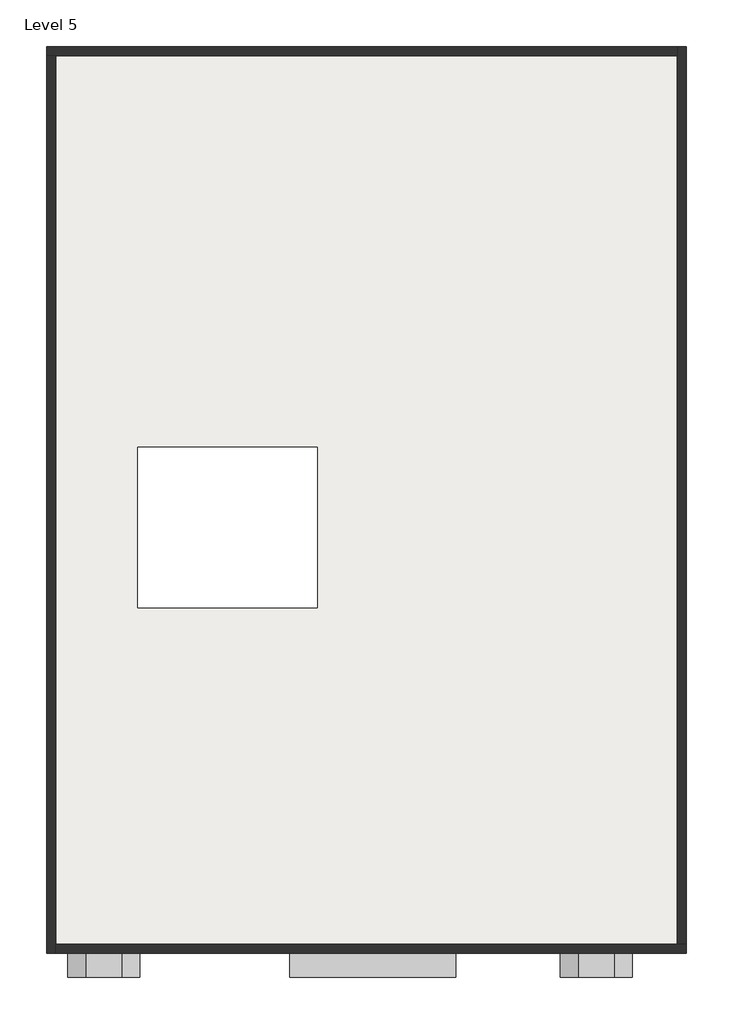
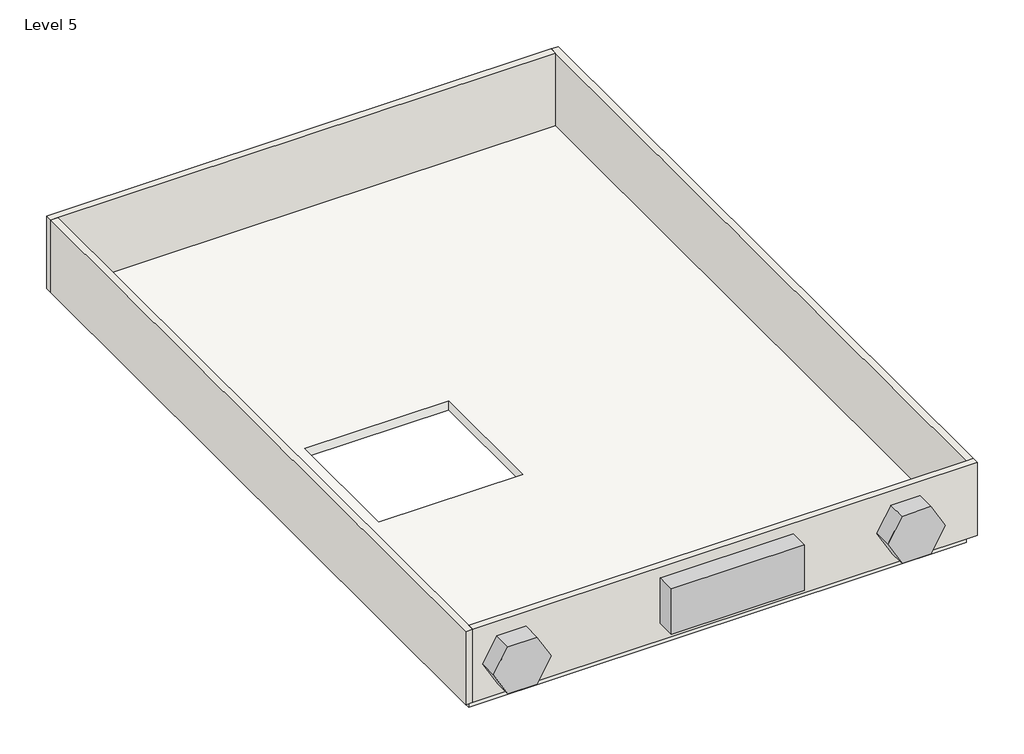
# One storey: 4 walls, 1 proxy, 1 roof.
"""IFC4 building model written with IfcOpenShell, lengths in millimetres."""

from ifc_helpers import new_model, si_unit, frame, origin, place, context, project, spatial, polyline, outline, extrude, faceted_brep, transform, mapped, element, save
from components import generic_models_1_generic_models_1_074ece3c

model = new_model("IFC4")

# Units and contexts
model_context = context("Model", 3, world=origin())
ifc_project = project(units=[si_unit("LENGTHUNIT", "METRE", prefix="MILLI")], contexts=[model_context])

# Site, building, storey
site = spatial("IfcSite", under=ifc_project)
building = spatial("IfcBuilding", under=site)
storey = spatial("IfcBuildingStorey", under=building, Name="Level 5", Elevation=9601.2)

# Proxy
placement = place(None, origin())
generic_models_1_generic_models_1_shape = generic_models_1_generic_models_1_074ece3c(model_context)
element("IfcBuildingElementProxy", 1, Name="Generic Models 1 : Generic Models 1", ObjectType="Generic Models 1 : Generic Models 1", at=placement, inside=storey, context=model_context, shape_type="MappedRepresentation", body=[
    mapped(generic_models_1_generic_models_1_shape, transform((0.0, 0.0, 0.0), x_axis=(1.0, 0.0, 0.0), y_axis=(0.0, 1.0, 0.0), z_axis=(0.0, 0.0, 1.0))),
])

# Roof
element("IfcRoof", 2, ObjectType="Generic - 12\"", at=placement, inside=storey, context=model_context, shape_type="SweptSolid", body=[
    extrude(outline(polyline([(-5216.1449167, -5508.2570853), (-5216.1449167, 5769.3429147), (2670.5550833, 5769.3429147), (2670.5550833, -5508.2570853), (-5216.1449167, -5508.2570853)]), holes=[polyline([(-1894.5382248, 797.2929147), (-4174.7449167, 797.2929147), (-4174.7449167, -1234.7070853), (-1894.5382248, -1234.7070853), (-1894.5382248, 797.2929147)])]), frame((0.0, 0.0, 9448.8), z_axis=(0.0, 0.0, 1.0), x_axis=(1.0, 0.0, 0.0)), (0.0, 0.0, 1.0), 152.4),
])

# Walls
element("IfcWall", 3, ObjectType="WALL4.5\"", at=placement, inside=storey, context=model_context, shape_type="Brep", body=[
    faceted_brep([(-5330.4449167, 5769.3429147, 9601.2), (-5216.1449167, 5769.3429147, 9601.2), (2670.5550833, 5769.3429147, 9601.2), (2670.5550833, 5769.3429147, 10820.4), (-5216.1449167, 5769.3429147, 10820.4), (-5330.4449167, 5769.3429147, 10820.4), (-5330.4449167, 5883.6429147, 9601.2), (-5330.4449167, 5883.6429147, 10820.4), (2670.5550833, 5883.6429147, 10820.4), (2670.5550833, 5883.6429147, 9601.2)], [[[0, 1, 2, 3, 4, 5]], [[6, 7, 8, 9]], [[2, 1, 0, 6, 9]], [[5, 4, 3, 8, 7]], [[0, 5, 7, 6]], [[3, 2, 9, 8]]]),
])
element("IfcWall", 4, ObjectType="WALL4.5\"", at=placement, inside=storey, context=model_context, shape_type="Brep", body=[
    faceted_brep([(-5216.1449167, -5622.5570853, 9601.2), (-5216.1449167, -5508.2570853, 9601.2), (-5216.1449167, 5769.3429147, 9601.2), (-5216.1449167, 5769.3429147, 10820.4), (-5216.1449167, -5508.2570853, 10820.4), (-5216.1449167, -5622.5570853, 10820.4), (-5330.4449167, -5622.5570853, 9601.2), (-5330.4449167, -5622.5570853, 10820.4), (-5330.4449167, 5769.3429147, 10820.4), (-5330.4449167, 5769.3429147, 9601.2)], [[[0, 1, 2, 3, 4, 5]], [[6, 7, 8, 9]], [[2, 1, 0, 6, 9]], [[5, 4, 3, 8, 7]], [[0, 5, 7, 6]], [[3, 2, 9, 8]]]),
])
element("IfcWall", 5, ObjectType="WALL4.5\"", at=placement, inside=storey, context=model_context, shape_type="Brep", body=[
    faceted_brep([(2784.8550833, -5508.2570853, 9601.2), (2670.5550833, -5508.2570853, 9601.2), (-5216.1449167, -5508.2570853, 9601.2), (-5216.1449167, -5508.2570853, 10820.4), (2670.5550833, -5508.2570853, 10820.4), (2784.8550833, -5508.2570853, 10820.4), (2784.8550833, -5622.5570853, 9601.2), (2784.8550833, -5622.5570853, 10820.4), (-5216.1449167, -5622.5570853, 10820.4), (-5216.1449167, -5622.5570853, 9601.2)], [[[0, 1, 2, 3, 4, 5]], [[6, 7, 8, 9]], [[2, 1, 0, 6, 9]], [[5, 4, 3, 8, 7]], [[0, 5, 7, 6]], [[3, 2, 9, 8]]]),
])
element("IfcWall", 6, ObjectType="WALL4.5\"", at=placement, inside=storey, context=model_context, shape_type="Brep", body=[
    faceted_brep([(2670.5550833, 5883.6429147, 9601.2), (2670.5550833, 5769.3429147, 9601.2), (2670.5550833, -5508.2570853, 9601.2), (2670.5550833, -5508.2570853, 10820.4), (2670.5550833, 5769.3429147, 10820.4), (2670.5550833, 5883.6429147, 10820.4), (2784.8550833, 5883.6429147, 9601.2), (2784.8550833, 5883.6429147, 10820.4), (2784.8550833, -5508.2570853, 10820.4), (2784.8550833, -5508.2570853, 9601.2)], [[[0, 1, 2, 3, 4, 5]], [[6, 7, 8, 9]], [[2, 1, 0, 6, 9]], [[5, 4, 3, 8, 7]], [[0, 5, 7, 6]], [[3, 2, 9, 8]]]),
])

save(model, "model.ifc")

# Revit data of these elements
# Type "Generic - 12\""
#   Assembly Code = "B1020"
#   Layers, outside or top first: 0' - 6" no material (function 1)
# Type "WALL4.5\""
#   Assembly Code = "B2010"
#   Layers, outside or top first: 0' - 4 1/2" "Parking Stripe" (function 1)
# Element 1 (IfcBuildingElementProxy, "Generic Models 1 : Generic Models 1")
#   Phase Created = New Construction
#   Materials on its faces: "Parking Stripe"
# Element 2 (IfcRoof, "Generic - 12\"")
#   built-in parameter 1001705 = 31.5 (stored number, unit not read)
#   built-in parameter 1001701 = -0.5 (stored number, unit not read)
#   built-in parameter 1001710 = 33615
#   Phase Created = New Construction
#   Materials on its faces: "Default Roof", "Wood Planks"
# Elements 3, 4, 5, 6 (IfcWall, "WALL4.5\"")
#   Top Offset = 0' - 0"
#   Base Offset = 0' - 0"
#   Unconnected Height = 4' - 0"
#   wall height = 4' - 0"
#   Phase Created = New Construction
#   Base Constraint = Level 5
#   Materials on its faces: "Parking Stripe", "Laminate, Ivory, Matte"
# Materials
#   "Parking Stripe": class "Paint", colour RGB 250 250 91, transparency 0, Cost = 0
#   "Default Roof": colour RGB 88 101 114, transparency 0, Cost = 0
#   "Wood Planks": class "Wood", colour RGB 193 160 115, transparency 0, Description = "Physical material.", Cost = 0
#   "Laminate, Ivory, Matte": class "Plastic", colour RGB 247 247 239, transparency 0, Description = "Plastic Laminate - Ivory, Matte", Cost = 0
